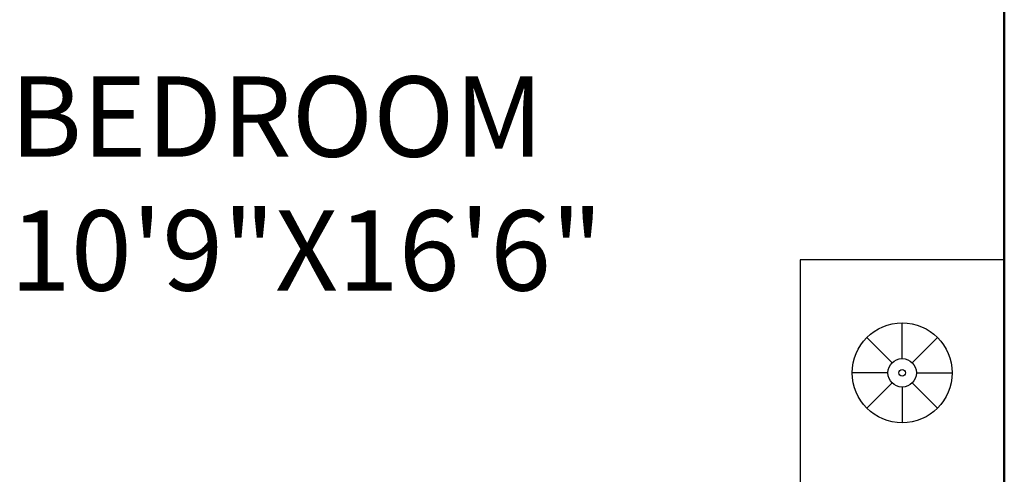
# Model space of a CAD drawing. Units: inches. Extents: x 3064 to 19385, y 846 to 15425.
# Tile 41 of 108: x 5240 to 5326, y 1090 to 1129. Entities that reach past the tile are written whole.
import ezdxf

# ---------------------------------------------------------------- set-up
doc = ezdxf.new("R2010")
doc.units = ezdxf.units.IN
for name, color, linetype, lineweight in [('A-AREA-IDEN', 3, 'Continuous', 18), ('A-FLOR-FIXT', 9, 'Continuous', 18), ('A-WALL', 7, 'Continuous', 50)]:
    doc.layers.add(name, color=color, linetype=linetype, lineweight=lineweight)
doc.layers.add('BLOCK', color=6, linetype='Continuous')
doc.styles.get("Standard").update_dxf_attribs({"font": 'arial.ttf'})

# ---------------------------------------------------------------- blocks, each defined once
blk = doc.blocks.new('A$C52E67D0D')
at = {"layer": 'BLOCK'}
for p, q in [((250.5, 1605.5), (250.5, 1684.7)), ((228.3, 1596.3), (172.3, 1652.3)), ((272.7, 1596.3), (328.7, 1652.3)), ((219.1, 1574.1), (139.9, 1574.1)), ((281.9, 1574.1), (361.1, 1574.1)), ((228.3, 1551.9), (172.3, 1495.9)), ((272.7, 1551.9), (328.7, 1495.9)), ((250.5, 1542.8), (250.5, 1463.5))]:
    blk.add_line(p, q, dxfattribs=at)
blk.add_lwpolyline([(501, 1348.6), (501, 1799.6), (0, 1799.6), (0, 1348.6)], close=True, dxfattribs=at)
for radius in [110.6, 31.4, 7.46]:
    blk.add_circle((250.5, 1574.1), radius, dxfattribs=at)

msp = doc.modelspace()

# ---------------------------------------------------------------- linework, layer by layer
at = {"layer": 'A-WALL'}
msp.add_line((5326.017, 1140.096), (5326.017, 978.096), dxfattribs=at)

# ---------------------------------------------------------------- block references
at = {"layer": 'A-FLOR-FIXT', "xscale": 0.039370099999992, "yscale": 0.039370099999992, "zscale": 0.039370099999992, "rotation": 270}
msp.add_blockref('A$C52E67D0D', (5255.151, 1108.348), dxfattribs=at)

# ---------------------------------------------------------------- texts
at = {"layer": 'A-AREA-IDEN', "insert": (5239.43, 1124.326), "char_height": 7, "attachment_point": 1}
msp.add_mtext_dynamic_manual_height_columns('BEDROOM\\P10\'9"X16\'6"', width=67.59241, gutter_width=12.5, heights=[0], dxfattribs=at)

doc.saveas('drawing.dxf')
